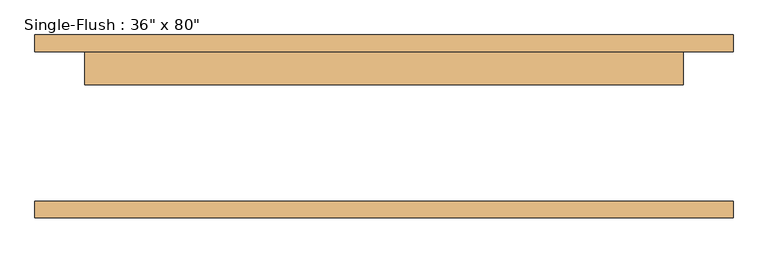
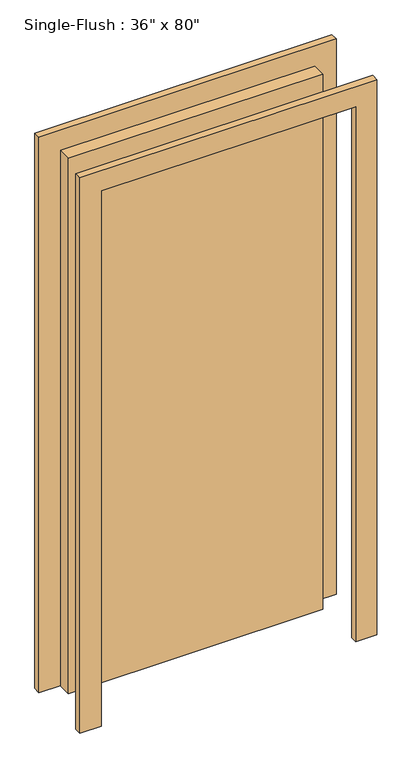
"""IFC4 building model written with IfcOpenShell, lengths in millimetres: door geometry."""

from ifc_helpers import new_model, si_unit, frame, origin, origin_with_axes, place, context, project, spatial, polyline, outline, extrude, source, transform, mapped, element, save


def door_89fc3733(model_context):
    return source(origin(), model_context, "Body", "SweptSolid", [
        extrude(outline(polyline([(2108.2, -533.4), (0.0, -533.4), (0.0, -457.2), (2032.0, -457.2), (2032.0, 457.2), (0.0, 457.2), (0.0, 533.4), (2108.2, 533.4), (2108.2, -533.4)])), frame((0.0, 114.3, 0.0), z_axis=(0.0, 1.0, 0.0), x_axis=(0.0, 0.0, 1.0)), (0.0, 0.0, 1.0), 25.4),
        extrude(outline(polyline([(2108.2, 533.4), (2108.2, -533.4), (0.0, -533.4), (0.0, -457.2), (2032.0, -457.2), (2032.0, 457.2), (0.0, 457.2), (0.0, 533.4), (2108.2, 533.4)])), frame((0.0, -139.7, 0.0), z_axis=(0.0, 1.0, 0.0), x_axis=(0.0, 0.0, 1.0)), (0.0, 0.0, 1.0), 25.4),
        extrude(outline(polyline([(457.2, 63.5), (-457.2, 63.5), (-457.2, 114.3), (457.2, 114.3), (457.2, 63.5)])), origin_with_axes(), (0.0, 0.0, 1.0), 2032.0),
    ])


if __name__ == "__main__":
    model = new_model("IFC4")
    model_context = context("Model", 3, world=origin())
    ifc_project = project(units=[si_unit("LENGTHUNIT", "METRE", prefix="MILLI")], contexts=[model_context])
    site = spatial("IfcSite", under=ifc_project)
    building = spatial("IfcBuilding", under=site)
    placement = place(None, origin())
    door_shape = door_89fc3733(model_context)
    element("IfcDoor", 1, ObjectType="Single-Flush : 36\" x 80\"", at=placement, inside=building, context=model_context, shape_type="MappedRepresentation", body=[
        mapped(door_shape, transform((0.0, 0.0, 0.0), x_axis=(1.0, 0.0, 0.0), y_axis=(0.0, 1.0, 0.0), z_axis=(0.0, 0.0, 1.0))),
    ])
    save(model, "model.ifc")

# Revit data of these elements
# Type "Single-Flush : 36\" x 80\""
#   Type Mark = "6"
#   Construction Type Id = "MDOOR"
#   Assembly Code = "C1020"
#   Analytic Construction = "Metal"
#   Thickness = 0' - 2"
#   Heat Transfer Coefficient (U) = 0.651978 BTU/(h·ft²·°F)
#   Height = 6' - 8"
#   Trim Projection Ext = 0' - 1"
#   Trim Projection Int = 0' - 1"
#   Trim Width = 0' - 3"
#   Width = 3' - 0"
#   Define Thermal Properties by = 1
#   Define Thermal Properties by = 1
#   Door Material = Door - Panel
#   Frame Material = Door - Frame
#   Visual Light Transmittance = 0
#   Solar Heat Gain Coefficient = 0
#   Function = (empty or 0)
#   Wall Closure = (empty or 0)
# Element 1 (IfcDoor, "Single-Flush : 36\" x 80\"")
#   Materials on its faces: "Door - Frame", "Door - Panel"
# Materials
#   "Door - Panel": class "Wood", colour RGB 210 159 95, transparency 0, Cost = 0
#   "Door - Frame": colour RGB 118 70 51, transparency 0, Cost = 0
